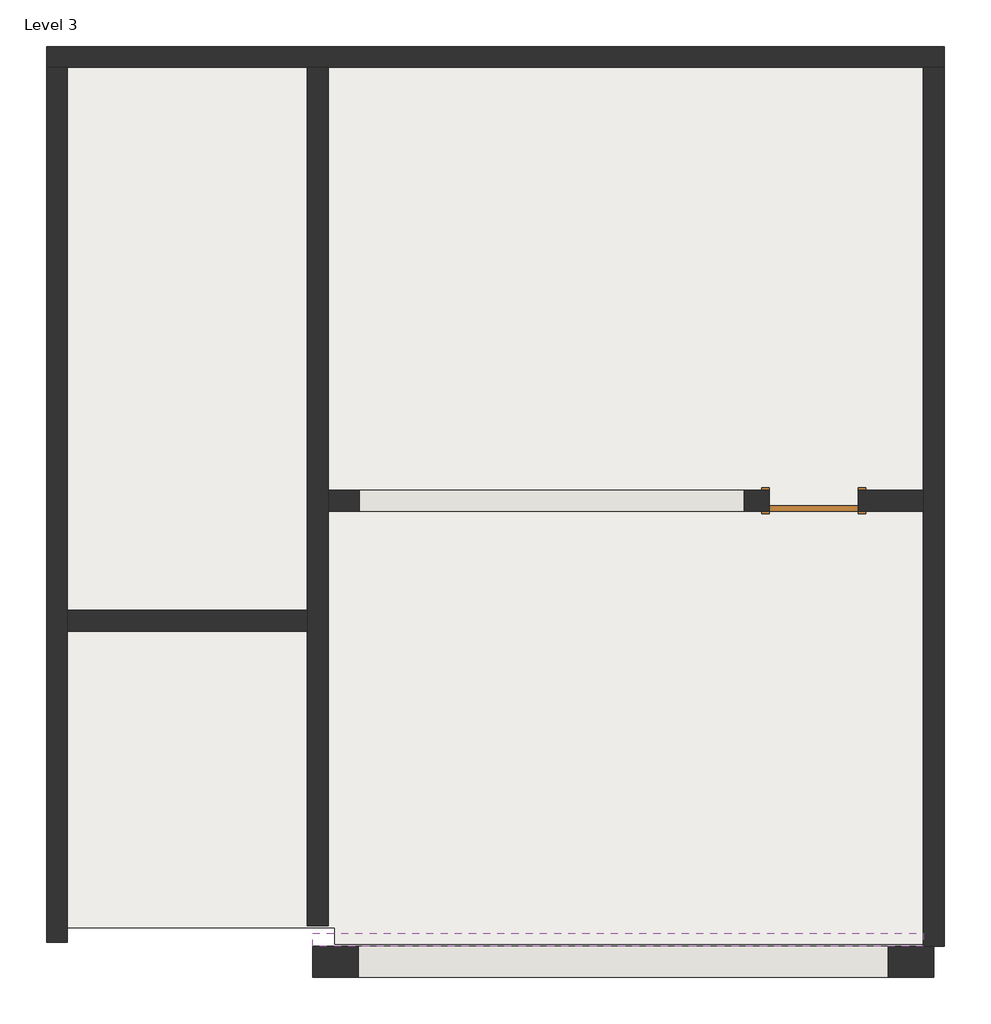
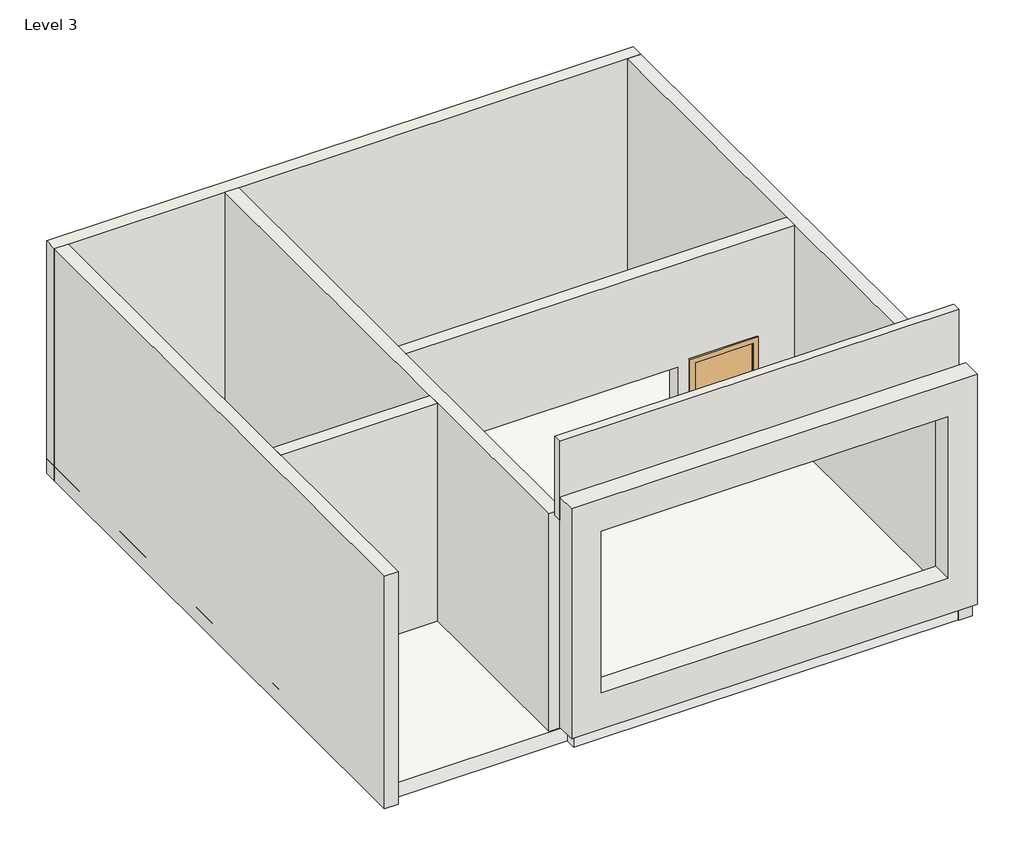
# One storey: 8 walls, 1 door, 1 roof.
"""IFC4 building model written with IfcOpenShell, lengths in millimetres."""

from ifc_helpers import new_model, si_unit, frame, origin, place, context, project, spatial, polyline, outline, extrude, faceted_brep, transform, mapped, element, save
from components import door_10fd3a06, walls_3_walls_1_396bf1f7

model = new_model("IFC4")

# Units and contexts
model_context = context("Model", 3, world=origin())
ifc_project = project(units=[si_unit("LENGTHUNIT", "METRE", prefix="MILLI")], contexts=[model_context])

# Site, building, storey
site = spatial("IfcSite", under=ifc_project)
building = spatial("IfcBuilding", under=site)
storey = spatial("IfcBuildingStorey", under=building, Name="Level 3", Elevation=8229.6)

# Door
placement = place(None, origin())
door_shape = door_10fd3a06(model_context)
element("IfcDoor", 1, ObjectType="Door-Single-Panel : 34\" x 80\"", at=placement, inside=storey, context=model_context, shape_type="MappedRepresentation", body=[
    mapped(door_shape, transform((-1366.3561565, 5783.1985991, 8229.6), x_axis=(-1.0, 0.0, 0.0), y_axis=(0.0, -1.0, 0.0), z_axis=(0.0, 0.0, 1.0))),
])

# Roof
element("IfcRoof", 2, ObjectType="Generic - 9\"", at=placement, inside=storey, context=model_context, shape_type="SweptSolid", body=[
    extrude(outline(polyline([(-8833.9561565, 10202.7985991), (-96.3561565, 10202.7985991), (-96.3561565, 1465.1985991), (-6027.2561565, 1465.1985991), (-6027.2561565, 1623.9485991), (-8833.9561565, 1623.9485991), (-8833.9561565, 10202.7985991)])), frame((0.0, 0.0, 8229.6), z_axis=(0.0, 0.0, 1.0), x_axis=(1.0, 0.0, 0.0)), (0.0, 0.0, 1.0), 228.6),
])

# Walls
element("IfcWall", 3, ObjectType="Generic - 5\"", at=placement, inside=storey, context=model_context, shape_type="SweptSolid", body=[
    extrude(outline(polyline([(-6243.1561565, 1573.1485991), (-299.5561565, 1573.1485991), (-299.5561565, 1446.1485991), (-6243.1561565, 1446.1485991), (-6243.1561565, 1573.1485991)])), frame((0.0, 0.0, 11891.0745283), z_axis=(0.0, 0.0, 1.0), x_axis=(1.0, 0.0, 0.0)), (0.0, 0.0, 1.0), 1240.7254717),
])
element("IfcWall", 4, ObjectType="Generic - 8\"", at=placement, inside=storey, context=model_context, shape_type="SweptSolid", body=[
    extrude(outline(polyline([(-6293.9561565, 4513.1985991), (-8630.7561565, 4513.1985991), (-8630.7561565, 4716.3985991), (-6293.9561565, 4716.3985991), (-6293.9561565, 4513.1985991)])), frame((0.0, 0.0, 8229.6), z_axis=(0.0, 0.0, 1.0), x_axis=(1.0, 0.0, 0.0)), (0.0, 0.0, 1.0), 3657.6),
])
element("IfcWall", 5, ObjectType="Generic - 8\"", at=placement, inside=storey, context=model_context, shape_type="Brep", body=[
    faceted_brep([(-6293.9561565, 9999.5985991, 8229.6), (-6293.9561565, 4716.3985991, 8229.6), (-6293.9561565, 4513.1985991, 8229.6), (-6293.9561565, 1642.9985991, 8229.6), (-6293.9561565, 1642.9985991, 11887.2), (-6293.9561565, 4513.1985991, 11887.2), (-6293.9561565, 4716.3985991, 11887.2), (-6293.9561565, 9999.5985991, 11887.2), (-6090.7561565, 9999.5985991, 8229.6), (-6090.7561565, 9999.5985991, 11887.2), (-6090.7561565, 5884.7985991, 11887.2), (-6090.7561565, 5681.5985991, 11887.2), (-6090.7561565, 1642.9985991, 11887.2), (-6090.7561565, 1642.9985991, 8229.6), (-6090.7561565, 5681.5985991, 8229.6), (-6090.7561565, 5884.7985991, 8229.6)], [[[0, 1, 2, 3, 4, 5, 6, 7]], [[8, 9, 10, 11, 12, 13, 14, 15]], [[3, 2, 1, 0, 8, 15, 14, 13]], [[4, 3, 13, 12]], [[7, 6, 5, 4, 12, 11, 10, 9]], [[0, 7, 9, 8]]]),
])
element("IfcWall", 6, ObjectType="Generic - 8\"", at=placement, inside=storey, context=model_context, shape_type="SweptSolid", body=[
    extrude(outline(polyline([(8229.6, -6090.7561565), (8229.6, -1798.1561565), (10261.6, -1798.1561565), (10261.6, -934.5561565), (8229.6, -934.5561565), (8229.6, -299.5561565), (11887.2, -299.5561565), (11887.2, -6090.7561565), (8229.6, -6090.7561565)]), holes=[polyline([(10256.008423, -2042.3901764), (8494.7392215, -2042.3901764), (8494.7392215, -5792.4012139), (10256.008423, -5792.4012139), (10256.008423, -2042.3901764)])]), frame((0.0, 5681.5985991, 0.0), z_axis=(0.0, 1.0, 0.0), x_axis=(0.0, 0.0, 1.0)), (0.0, 0.0, 1.0), 203.2),
])
element("IfcWall", 7, ObjectType="Generic - 8\"", at=placement, inside=storey, context=model_context, shape_type="Brep", body=[
    faceted_brep([(-8833.9561565, 9999.5985991, 8229.6), (-8630.7561565, 9999.5985991, 8229.6), (-6293.9561565, 9999.5985991, 8229.6), (-6090.7561565, 9999.5985991, 8229.6), (-299.5561565, 9999.5985991, 8229.6), (-96.3561565, 9999.5985991, 8229.6), (-96.3561565, 9999.5985991, 11887.2), (-299.5561565, 9999.5985991, 11887.2), (-6090.7561565, 9999.5985991, 11887.2), (-6293.9561565, 9999.5985991, 11887.2), (-8630.7561565, 9999.5985991, 11887.2), (-8833.9561565, 9999.5985991, 11887.2), (-8833.9561565, 10202.7985991, 8229.6), (-8833.9561565, 10202.7985991, 11887.2), (-96.3561565, 10202.7985991, 11887.2), (-96.3561565, 10202.7985991, 8229.6)], [[[0, 1, 2, 3, 4, 5, 6, 7, 8, 9, 10, 11]], [[12, 13, 14, 15]], [[5, 4, 3, 2, 1, 0, 12, 15]], [[11, 10, 9, 8, 7, 6, 14, 13]], [[6, 5, 15, 14]], [[0, 11, 13, 12]]]),
])
element("IfcWall", 8, ObjectType="Generic - 8\"", at=placement, inside=storey, context=model_context, shape_type="Brep", body=[
    faceted_brep([(-299.5561565, 9999.5985991, 8229.6), (-299.5561565, 5884.7985991, 8229.6), (-299.5561565, 5681.5985991, 8229.6), (-299.5561565, 1446.1485991, 8229.6), (-299.5561565, 1446.1485991, 9201.3855951), (-299.5561565, 1446.1485991, 11887.2), (-299.5561565, 1465.1985991, 11887.2), (-299.5561565, 5681.5985991, 11887.2), (-299.5561565, 5884.7985991, 11887.2), (-299.5561565, 9999.5985991, 11887.2), (-96.3561565, 9999.5985991, 8229.6), (-96.3561565, 9999.5985991, 11887.2), (-96.3561565, 1465.1985991, 11887.2), (-96.3561565, 1446.1485991, 11887.2), (-96.3561565, 1446.1485991, 8229.6)], [[[0, 1, 2, 3, 4, 5, 6, 7, 8, 9]], [[10, 11, 12, 13, 14]], [[3, 2, 1, 0, 10, 14]], [[6, 5, 13, 12]], [[9, 8, 7, 6, 12, 11]], [[5, 4, 3, 14, 13]], [[0, 9, 11, 10]]]),
])
element("IfcWall", 9, ObjectType="Generic - 8\"", at=placement, inside=storey, context=model_context, shape_type="Brep", body=[
    faceted_brep([(-8630.7561565, 1484.2485991, 8229.6), (-8630.7561565, 4513.1985991, 8229.6), (-8630.7561565, 4716.3985991, 8229.6), (-8630.7561565, 9999.5985991, 8229.6), (-8630.7561565, 9999.5985991, 11887.2), (-8630.7561565, 4716.3985991, 11887.2), (-8630.7561565, 4513.1985991, 11887.2), (-8630.7561565, 1484.2485991, 11887.2), (-8833.9561565, 1484.2485991, 8229.6), (-8833.9561565, 1484.2485991, 11887.2), (-8833.9561565, 9999.5985991, 11887.2), (-8833.9561565, 9999.5985991, 8229.6)], [[[0, 1, 2, 3, 4, 5, 6, 7]], [[8, 9, 10, 11]], [[3, 2, 1, 0, 8, 11]], [[7, 6, 5, 4, 10, 9]], [[0, 7, 9, 8]], [[4, 3, 11, 10]]]),
])
walls_3_walls_1_shape = walls_3_walls_1_396bf1f7(model_context)
element("IfcWall", 10, ObjectType="Walls 3 : Walls 1", at=placement, inside=storey, context=model_context, shape_type="MappedRepresentation", body=[
    mapped(walls_3_walls_1_shape, transform((0.0, 0.0, 0.0), x_axis=(1.0, 0.0, 0.0), y_axis=(0.0, 1.0, 0.0), z_axis=(0.0, 0.0, 1.0))),
])

save(model, "model.ifc")

# Revit data of these elements
# Type "Door-Single-Panel : 34\" x 80\""
#   Type Mark = "8"
#   Construction Type Id = "DOOR"
#   Assembly Code = "C1020300"
#   Analytic Construction = "Wooden"
#   Thickness = 0' - 2"
#   Thermal Resistance (R) = 2.5876 (h·ft²·°F)/BTU
#   Swing Angle [instance default] = 90.00°
#   Heat Transfer Coefficient (U) = 0.3865 BTU/(h·ft²·°F)
#   Height = 6' - 8"
#   Trim Projection Ext = 0' - 1"
#   Trim Projection Int = 0' - 1"
#   Trim Width = 0' - 3"
#   Width = 2' - 10"
#   Define Thermal Properties by = 1
#   Panel Material = Wood - Birch - Solid Stained Light Low Gloss
#   Trim Material = Paint - Sienna
#   Visual Light Transmittance = 0
#   Solar Heat Gain Coefficient = 0
#   Function = (empty or 0)
#   Wall Closure = (empty or 0)
# Type "Generic - 9\""
#   Assembly Code = "B1020"
#   Layers, outside or top first: 0' - 9" no material (function 1)
# Type "Generic - 5\""
#   Assembly Code = "B2010"
#   Layers, outside or top first: 0' - 5" no material (function 1)
# Type "Generic - 8\""
#   Assembly Code = "B2010"
#   Layers, outside or top first: 0' - 8" no material (function 1)
# Element 1 (IfcDoor, "Door-Single-Panel : 34\" x 80\"")
#   Swing Angle = 90.00°
#   Phase Created = New Construction
#   Materials on its faces: "Paint - Sienna", "Wood - Birch - Solid Stained Light Low Gloss"
# Element 2 (IfcRoof, "Generic - 9\"")
#   built-in parameter 1001705 = 27.75 (stored number, unit not read)
#   built-in parameter 1001710 = 33615
#   Phase Created = New Construction
#   Materials on its faces: "Default Roof"
# Element 3 (IfcWall, "Generic - 5\"")
#   built-in parameter 1001111 = 12' - 0.15254"
#   Top Offset = 4' - 1"
#   Base Offset = 12' - 0.15254"
#   wall height = 4' - 0.84746"
#   Phase Created = New Construction
#   Base Constraint = Level 3
#   Top Constraint = Level 4
#   Materials on its faces: "Default Wall"
# Elements 4, 5, 6, 7, 8, 9 (IfcWall, "Generic - 8\"")
#   Top Offset = 0' - 0"
#   Base Offset = 0' - 0"
#   Unconnected Height = 12' - 0"
#   wall height = 12' - 0"
#   Phase Created = New Construction
#   Base Constraint = Level 3
#   Materials on its faces: "Default Wall"
# Element 10 (IfcWall, "Walls 3 : Walls 1")
#   Phase Created = New Construction
#   Materials on its faces: "Default Wall"
# Materials
#   "Wood - Birch - Solid Stained Light Low Gloss": class "Wood", colour RGB 210 159 95, transparency 0, Cost = 0
#   "Paint - Sienna": colour RGB 118 70 51, transparency 0, Cost = 0
#   "Default Roof": colour RGB 88 101 114, transparency 0
#   "Default Wall": colour RGB 128 128 128, transparency 0
